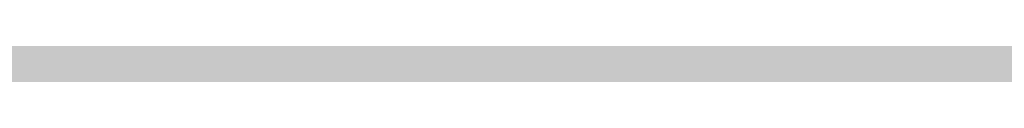
# Model space of a CAD drawing. Units: inches. Extents: x 2091 to 2899, y 967 to 2217.
# Tile 199 of 256: x 2203.18039 to 2203.25707, y 1152.24874 to 1152.25042. Entities that reach past the tile are written whole.
import ezdxf

# ---------------------------------------------------------------- set-up
doc = ezdxf.new("R2010")
doc.units = ezdxf.units.IN
doc.layers.add('A-WALL-PATT', color=141, linetype='Continuous', lineweight=13, true_color=0xadddf7)

msp = doc.modelspace()

# ---------------------------------------------------------------- hatches: boundary and pattern name
at = {"layer": 'A-WALL-PATT'}
h = msp.add_hatch(color=256, dxfattribs=at)
h.dxf.hatch_style = 1
h.paths.add_polyline_path([(2803.143603, 2050.919059), (2203.143603, 2050.919059), (2203.143603, 1090.919059), (2803.143603, 1090.919059)])
h.paths.add_polyline_path([(2635.79885, 1147.540465), (2674.524052, 1147.540465, 0.376086), (2678.529665, 1152.880202), (2678.529665, 1159.556473, 0.333335), (2674.524319, 1163.561846), (2674.524319, 1163.56185), (2674.524319, 1192.93439), (2635.805971, 1192.93439), (2597.087622, 1192.93439), (2597.087622, 1163.561846, 0.333335), (2593.082276, 1159.556473), (2593.082276, 1152.880202, 0.376086), (2597.087889, 1147.540465)], flags=0)
h.paths.add_polyline_path([(2436.010433, 1278.240778, 0.000483), (2435.952643, 1278.215027, -0.001328), (2435.935625, 1278.111693, -0.001711), (2436.11644, 1278.040758, 0.002185)], flags=0)
h.paths.add_polyline_path([(2794.143603, 1143.419059), (2794.143603, 1347.419059), (2543.370171, 1347.419059), (2543.370171, 1351.919059), (2794.143603, 1351.919059), (2794.143603, 1392.713555), (2793.947398, 1392.713555), (2793.947398, 1473.5369), (2794.143603, 1473.5369), (2794.143603, 1531.919059), (2650.143603, 1531.919059), (2650.143603, 1536.419059), (2794.143603, 1536.419059), (2794.143603, 1692.419059), (2609.375609, 1692.419059), (2609.375609, 1644.419059), (2604.875609, 1644.419059), (2604.875609, 1744.919059), (2609.375609, 1744.919059), (2609.375609, 1696.919059), (2794.143603, 1696.919059), (2794.143603, 1780.919059), (2609.643603, 1780.919059), (2493.875609, 1780.919059), (2493.875609, 1785.419059), (2609.643603, 1785.419059), (2794.143603, 1785.419059), (2794.143603, 1847.938821), (2793.951222, 1847.938821), (2793.951222, 1928.762166), (2794.143603, 1928.762166), (2794.143603, 1941.419059), (2614.143603, 1941.419059), (2614.143603, 1821.419059), (2609.643603, 1821.419059), (2609.643603, 1941.419059), (2392.143603, 1941.419059), (2392.143603, 1819.919059), (2387.643603, 1819.919059), (2387.643603, 1941.419059), (2212.143603, 1941.419059), (2212.143603, 1783.919059), (2392.143603, 1783.919059), (2392.143603, 1780.919059), (2212.143603, 1780.919059), (2212.143603, 1629.419059), (2387.643603, 1629.419059), (2387.643603, 1744.919059), (2392.143603, 1744.919059), (2392.143603, 1627.919059), (2317.143603, 1627.919059), (2317.143603, 1551.419059), (2317.143603, 1536.419059), (2459.383591, 1536.419059), (2459.383591, 1602.39648), (2463.883591, 1602.39648), (2463.883591, 1531.919059), (2456.643603, 1531.919059), (2456.643603, 1529.919059), (2452.143603, 1529.919059), (2452.143603, 1531.919059), (2312.643603, 1531.919059), (2312.643603, 1551.419059), (2306.143603, 1551.419059), (2306.143603, 1555.919059), (2308.143603, 1555.919059), (2308.143603, 1551.419059), (2312.643603, 1551.419059), (2312.643603, 1627.919059), (2212.143603, 1627.919059), (2212.143603, 1555.919059), (2270.143603, 1555.919059), (2270.143603, 1551.419059), (2212.143603, 1551.419059), (2212.143603, 1351.919059), (2272.143603, 1351.919059), (2272.143603, 1347.419059), (2212.143603, 1347.419059), (2212.143603, 1275.419059), (2308.143603, 1275.419059), (2308.143603, 1351.919059), (2452.143603, 1351.919059), (2452.143603, 1493.919059), (2456.643603, 1493.919059), (2456.643603, 1347.419059), (2312.643603, 1347.419059), (2312.643603, 1270.919059), (2212.143603, 1270.919059), (2212.143603, 1099.919059), (2281.237523, 1099.919059), (2282.871041, 1110.913803), (2282.008341, 1116.996603), (2278.557741, 1121.420403), (2268.205641, 1128.056203), (2272.087641, 1128.056203), (2273.812941, 1131.927003), (2279.420341, 1134.691903), (2285.027841, 1135.244903), (2287.615841, 1137.456803), (2288.047141, 1138.009803), (2289.341141, 1140.774703), (2291.066541, 1139.668703), (2292.360541, 1135.244903), (2295.379841, 1136.903803), (2296.242541, 1135.797903), (2297.105241, 1133.033003), (2300.124641, 1138.009803), (2303.143941, 1138.009803), (2304.437941, 1135.797903), (2303.143941, 1133.586003), (2306.594641, 1134.691903), (2307.888741, 1133.033003), (2310.908041, 1135.244903), (2313.927441, 1134.138903), (2315.62686, 1132.427102), (2308.320041, 1117.549603), (2290.203841, 1109.807903), (2288.909841, 1103.172103), (2289.272309, 1099.919059), (2434.918227, 1099.919059), (2431.593227, 1124.788059), (2429.930227, 1169.553059), (2430.927185, 1240.519694), (2435.658926, 1238.186126), (2437.135227, 1196.554059), (2438.798227, 1143.973059), (2442.678227, 1111.998059), (2446.558227, 1099.919059), (2794.143603, 1099.919059), (2794.143603, 1138.919059), (2548.032447, 1138.919059), (2548.032447, 1143.419059), (2548.032447, 1148.819059), (2546.668457, 1148.031559), (2528.685692, 1179.178622, 0.256256), (2512.032447, 1148.819059), (2512.032447, 1143.419059), (2512.032447, 1138.919059), (2507.532447, 1138.919059), (2507.532447, 1143.419059), (2507.532447, 1148.819059, 0.256256), (2490.879202, 1179.178622), (2472.896437, 1148.031559), (2471.532447, 1148.819059), (2471.532447, 1143.419059), (2467.032447, 1143.419059), (2467.032447, 1269.945786, 0.039061), (2460.909987, 1273.580059), (2467.032447, 1273.580059), (2467.032447, 1286.325364, 0.014511), (2465.216194, 1286.761905), (2467.032447, 1287.052576), (2467.032447, 1323.419059), (2471.532447, 1323.419059), (2471.532447, 1148.819059), (2489.532447, 1179.995973), (2490.896437, 1179.208473), (2490.879202, 1179.178622, -0.256256), (2507.532447, 1148.819059), (2507.532447, 1143.419059), (2512.032447, 1143.419059), (2512.032447, 1148.819059, -0.256256), (2528.685692, 1179.178622), (2528.668457, 1179.208473), (2530.032447, 1179.995973), (2548.032447, 1148.819059), (2548.032447, 1143.419059)], flags=16)
h.paths.add_polyline_path([(2607.768546, 1200.945083), (2607.768546, 1265.030625), (2597.087622, 1281.052011), (2619.784585, 1281.052011), (2627.795278, 1337.12686), (2635.79885, 1337.12686), (2643.816663, 1337.12686), (2651.827356, 1281.052011), (2674.524319, 1281.052011), (2663.843395, 1265.030625), (2663.843395, 1200.945083), (2635.805971, 1200.945083)], flags=0)
edge = h.paths.add_edge_path(flags=0)
edge.add_ellipse((13303.896215, 1272.998725), major_axis=(-10595.31304, 0.000001), ratio=0.842303870086, start_angle=0.6282372191, end_angle=0.6465540999, ccw=False)
edge.add_ellipse((2711.70045, 1156.852678), major_axis=(2.219769, 0), ratio=0.84230387, start_angle=111.535244, end_angle=180.628237, ccw=False)
edge.add_ellipse((13303.156292, 1272.998725), major_axis=(-10593.026306, 0), ratio=0.842303869544, start_angle=0.5282714718, end_angle=0.6465540971, ccw=False)
edge.add_line((2710.764596, 1175.333295), (2710.129986, 1175.333295))
edge.add_ellipse((2710.129986, 1176.579775), major_axis=(1.479846, 0), ratio=0.84230387, start_angle=180, end_angle=270, ccw=False)
edge.add_line((2708.65014, 1176.579775), (2708.65014, 1200.782914))
edge.add_ellipse((2710.129986, 1200.782914), major_axis=(1.479846, 0), ratio=0.84230387, start_angle=90, end_angle=180, ccw=False)
edge.add_line((2710.129986, 1202.029394), (2710.465075, 1202.029394))
edge.add_ellipse((13303.156292, 1272.998725), major_axis=(-10593.026306, 0), ratio=0.842303869544, start_angle=-0.0902290886, end_angle=0.3838667788, ccw=False)
edge.add_ellipse((2710.129986, 1290.927031), major_axis=(-1.479846, 0), ratio=0.84230387, start_angle=0, end_angle=90, ccw=False)
edge.add_line((2708.65014, 1290.927031), (2708.65014, 1315.13017))
edge.add_ellipse((2710.129986, 1315.13017), major_axis=(-1.479846, 0), ratio=0.84230387, start_angle=-90, end_angle=0, ccw=False)
edge.add_line((2710.129986, 1316.37665), (2710.706314, 1316.37665))
edge.add_ellipse((3238.40172, 1296.289566), major_axis=(528.234, 0), ratio=0.8423038695, start_angle=176.34957241, end_angle=177.82004969, ccw=False)
edge.add_ellipse((2775.063043, 1071.450696), major_axis=(313.307761, 0), ratio=0.8423038695, start_angle=102.12596555, end_angle=103.78052899, ccw=False)
edge.add_ellipse((2775.063043, 1078.305698), major_axis=(-305.302891, 0), ratio=0.8423038695, start_angle=-79.790461, end_angle=-77.55537271, ccw=False)
edge.add_ellipse((2695.141767, 1541.975383), major_axis=(-250.960216, 0), ratio=0.8423038695, start_angle=99.25656601, end_angle=102.55493264)
edge.add_line((2741.410326, 1334.214255), (2747.132545, 1337.378477))
edge.add_ellipse((2747.538616, 1336.857478), major_axis=(-0.739923, 0), ratio=0.8423039, start_angle=270, end_angle=307.93313, ccw=False)
edge.add_ellipse((2747.538616, 1336.857478), major_axis=(-0.739923, 0), ratio=0.8423039, start_angle=232.06687, end_angle=270, ccw=False)
edge.add_line((2747.944687, 1337.378477), (2753.666906, 1334.214255))
edge.add_ellipse((2799.935466, 1541.975383), major_axis=(250.960216, 0), ratio=0.8423038695, start_angle=257.44506736, end_angle=260.74343399)
edge.add_ellipse((2720.014189, 1078.305698), major_axis=(305.302891, 0), ratio=0.8423038695, start_angle=77.55537271, end_angle=79.790461, ccw=False)
edge.add_ellipse((2720.014189, 1071.450696), major_axis=(-313.307761, 0), ratio=0.8423038695, start_angle=256.21947101, end_angle=257.87403445, ccw=False)
edge.add_ellipse((2256.675512, 1296.289566), major_axis=(-528.234, 0), ratio=0.8423038695, start_angle=182.17995031, end_angle=183.65042759, ccw=False)
edge.add_line((2784.370918, 1316.37665), (2784.947247, 1316.37665))
edge.add_ellipse((2784.947247, 1315.13017), major_axis=(1.479846, 0), ratio=0.84230387, start_angle=0, end_angle=90, ccw=False)
edge.add_line((2786.427093, 1315.13017), (2786.427093, 1290.927031))
edge.add_ellipse((2784.947247, 1290.927031), major_axis=(1.479846, 0), ratio=0.84230387, start_angle=270, end_angle=360, ccw=False)
edge.add_ellipse((-7808.07906, 1272.998725), major_axis=(10593.026306, 0), ratio=0.842303869544, start_angle=-0.3838667788, end_angle=0.0902290886, ccw=False)
edge.add_line((2784.612157, 1202.029394), (2784.947247, 1202.029394))
edge.add_ellipse((2784.947247, 1200.782914), major_axis=(1.479846, 0), ratio=0.84230387, start_angle=0, end_angle=90, ccw=False)
edge.add_line((2786.427093, 1200.782914), (2786.427093, 1176.579775))
edge.add_ellipse((2784.947247, 1176.579775), major_axis=(-1.479846, 0), ratio=0.84230387, start_angle=90, end_angle=180, ccw=False)
edge.add_line((2784.947247, 1175.333295), (2784.312636, 1175.333295))
edge.add_ellipse((-7808.07906, 1272.998725), major_axis=(10593.026306, 0), ratio=0.842303869544, start_angle=-0.6186431963, end_angle=-0.5282714718, ccw=False)
edge.add_ellipse((2783.376783, 1156.852678), major_axis=(-2.219769, 0), ratio=0.84230387, start_angle=179.371763, end_angle=248.464757, ccw=False)
edge.add_ellipse((-7808.818983, 1272.998725), major_axis=(-10595.31304, 0.000004), ratio=0.842303865762, start_angle=179.3534459226, end_angle=179.3717628034, ccw=False)
edge.add_ellipse((2780.297303, 1153.500793), major_axis=(-5.246426, 0), ratio=0.84230387, start_angle=90, end_angle=179.353446, ccw=False)
edge.add_line((2780.297303, 1149.081708), (2714.77993, 1149.081708))
edge.add_ellipse((2714.77993, 1153.500793), major_axis=(5.246426, 0), ratio=0.84230387, start_angle=180.646554, end_angle=270, ccw=False)
edge = h.paths.add_edge_path(flags=0)
edge.add_line((2718.187367, 1151.007833), (2718.187367, 1170.472364))
edge.add_ellipse((2721.14706, 1170.472364), major_axis=(-2.959692, 0), ratio=0.84230387, start_angle=-90, end_angle=0, ccw=False)
edge.add_line((2721.14706, 1172.965324), (2773.930173, 1172.965324))
edge.add_ellipse((2773.930173, 1170.472364), major_axis=(-2.959692, 0), ratio=0.84230387, start_angle=180, end_angle=270, ccw=False)
edge.add_line((2776.889865, 1170.472364), (2776.889865, 1151.007833))
edge.add_line((2776.889865, 1151.007833), (2718.187367, 1151.007833))
edge = h.paths.add_edge_path(flags=0)
edge.add_line((2718.187367, 1180.23415), (2718.187367, 1199.057834))
edge.add_ellipse((2747.538616, 1320.39864), major_axis=(147.017924, 0), ratio=0.8423038695, start_angle=256.40186531, end_angle=283.59813469)
edge.add_line((2776.889865, 1199.057834), (2776.889865, 1180.23415))
edge.add_ellipse((2747.538616, 1301.574956), major_axis=(147.017924, 0), ratio=0.8423038695, start_angle=256.40186531, end_angle=283.59813469, ccw=False)
edge = h.paths.add_edge_path(flags=0)
edge.add_ellipse((13303.156292, 1272.998725), major_axis=(-10591.54646, 0), ratio=0.842303869555, start_angle=0.0555943135, end_angle=0.3777641939, ccw=False)
edge.add_line((2711.616859, 1262.72171), (2715.667408, 1249.495396))
edge.add_ellipse((6413.891963, 1241.691919), major_axis=(-3698.236159, 0), ratio=0.84230386955, start_angle=-0.120897369, end_angle=0.364076349)
edge.add_line((2715.761038, 1218.192455), (2711.934307, 1203.167361))
edge = h.paths.add_edge_path(flags=0)
edge.add_line((2718.187367, 1251.074566), (2716.002485, 1267.450435))
edge.add_ellipse((2742.151175, 1202.18954), major_axis=(81.772585, 0), ratio=0.84230387, start_angle=94.27742096, end_angle=111.8349538, ccw=False)
edge.add_line((2737.009748, 1270.930626), (2758.067484, 1270.930626))
edge.add_ellipse((2752.926058, 1202.18954), major_axis=(81.772585, 0), ratio=0.84230387, start_angle=68.1650462, end_angle=85.72257904, ccw=False)
edge.add_line((2779.074747, 1267.450435), (2776.889865, 1251.074566))
edge.add_ellipse((2750.338059, 1187.885356), major_axis=(79.579664, 0), ratio=0.84230387, start_angle=67.20808512, end_angle=85.1299304)
edge.add_line((2756.034656, 1254.743656), (2739.042576, 1254.743656))
edge.add_ellipse((2744.739174, 1187.885356), major_axis=(79.579664, 0), ratio=0.84230387, start_angle=94.8700696, end_angle=112.79191488)
edge = h.paths.add_edge_path(flags=0)
edge.add_line((2783.142926, 1203.167361), (2779.316194, 1218.192455))
edge.add_ellipse((-918.81473, 1241.691919), major_axis=(3698.236159, 0), ratio=0.84230386955, start_angle=-0.364076349, end_angle=0.120897369)
edge.add_line((2779.409825, 1249.495396), (2783.460373, 1262.72171))
edge.add_ellipse((-7808.07906, 1272.998725), major_axis=(-10591.54646, 0), ratio=0.84230386954, start_angle=179.6222358061, end_angle=179.9444056865, ccw=False)
edge = h.paths.add_edge_path(flags=0)
edge.add_ellipse((2734.200892, 1286.69044), major_axis=(-0.356609, 6.340078), ratio=0.60383358, start_angle=89.0020143, end_angle=253.657408, ccw=False)
edge.add_line((2730.369001, 1286.541806), (2730.369001, 1301.35198))
edge.add_line((2730.369001, 1301.35198), (2735.913311, 1305.214803))
edge.add_ellipse((2736.384917, 1304.734561), major_axis=(0.739923, 0), ratio=0.8423039, start_angle=90, end_angle=134.480211, ccw=False)
edge.add_line((2736.384917, 1305.357801), (2738.032783, 1305.357801))
edge.add_line((2738.032783, 1305.357801), (2738.032783, 1307.707927))
edge.add_ellipse((2794.201642, 1307.707927), major_axis=(56.168859, 0), ratio=0.84230387, start_angle=150.5614304, end_angle=180, ccw=False)
edge.add_ellipse((2700.875591, 1307.707927), major_axis=(-56.168859, 0), ratio=0.84230387, start_angle=180, end_angle=209.4385696, ccw=False)
edge.add_line((2757.04445, 1307.707927), (2757.04445, 1305.357801))
edge.add_line((2757.04445, 1305.357801), (2758.692316, 1305.357801))
edge.add_ellipse((2758.692316, 1304.734561), major_axis=(-0.739923, 0), ratio=0.8423039, start_angle=225.519789, end_angle=270, ccw=False)
edge.add_line((2759.163922, 1305.214803), (2764.708231, 1301.35198))
edge.add_line((2764.708231, 1301.35198), (2764.708231, 1286.541806))
edge.add_ellipse((2760.87634, 1286.69044), major_axis=(0.356609, 6.340078), ratio=0.60383358, start_angle=106.342592, end_angle=270.9979857, ccw=False)
edge.add_line((2757.04445, 1285.79709), (2757.04445, 1307.707927))
edge.add_ellipse((2700.875591, 1307.707927), major_axis=(-56.168859, 0), ratio=0.84230387, start_angle=180, end_angle=209.4385696)
edge.add_ellipse((2794.201642, 1307.707927), major_axis=(56.168859, 0), ratio=0.84230387, start_angle=150.5614304, end_angle=180)
edge.add_line((2738.032783, 1307.707927), (2738.032783, 1285.79709))
h.paths.add_polyline_path([(2417.812273, 1104.449704), (2413.492273, 1102.529704), (2410.612273, 1103.969704), (2409.172273, 1106.369704), (2407.252273, 1107.329704), (2406.292273, 1109.729704), (2405.332273, 1114.049704), (2405.332273, 1117.889704), (2406.292273, 1120.129704), (2407.252273, 1119.809704), (2408.848322, 1118.327658), (2410.173945, 1119.42417), (2410.211273, 1120.405704), (2411.040731, 1121.419054), (2410.699273, 1119.858704), (2410.173945, 1119.42417), (2410.088452, 1117.176109), (2411.132836, 1116.206324), (2413.972273, 1119.329704), (2416.852273, 1120.769704), (2416.869721, 1120.798784), (2417.035071, 1119.405116), (2417.896213, 1118.143384), (2418.292273, 1118.369704), (2419.544447, 1120.039269), (2419.360915, 1118.387487), (2419.032108, 1119.356151), (2418.398939, 1118.511926), (2419.252273, 1114.529704), (2418.794091, 1107.198795)], flags=0)
h.paths.add_polyline_path([(2508.870171, 1347.419059), (2508.370171, 1347.419059), (2508.370171, 1351.919059), (2508.870171, 1351.919059)], flags=0)
h.paths.add_polyline_path([(2473.370171, 1347.419059), (2472.370171, 1347.419059), (2467.870171, 1347.419059), (2467.870171, 1455.419059), (2472.370171, 1455.419059), (2472.370171, 1352.419059), (2473.370171, 1352.419059)], flags=0)
h.paths.add_polyline_path([(2352.106244, 1217.446197), (2349.226244, 1218.886197), (2347.786244, 1221.286197), (2345.866244, 1222.246197), (2344.906244, 1224.646197), (2343.946244, 1228.966197), (2343.946244, 1232.806197), (2344.906244, 1235.046197), (2345.866244, 1234.726197), (2347.462293, 1233.244152), (2348.787916, 1234.340663), (2348.825244, 1235.322197), (2349.654702, 1236.335547), (2349.313244, 1234.775197), (2348.787916, 1234.340663), (2348.702423, 1232.092603), (2349.746807, 1231.122817), (2352.586244, 1234.246197), (2355.466244, 1235.686197), (2355.483692, 1235.715277), (2355.649043, 1234.321609), (2356.510185, 1233.059877), (2356.906244, 1233.286197), (2358.158418, 1234.955762), (2357.974887, 1233.30398), (2357.646079, 1234.272644), (2357.012911, 1233.428419), (2357.866244, 1229.446197), (2357.408062, 1222.115288), (2356.426244, 1219.366197)], flags=0)
h.paths.add_polyline_path([(2348.2968, 1112.22442), (2347.0138, 1112.31042), (2345.5298, 1114.12742), (2345.7318, 1115.85842), (2346.8118, 1116.98242), (2346.8118, 1114.64642), (2345.8668, 1114.21442), (2346.8798, 1114.30042)], flags=0)
h.paths.add_polyline_path([(2347.0138, 1110.92642), (2346.2718, 1110.49342), (2346.6098, 1111.18642)], flags=0)
h.paths.add_polyline_path([(2345.8668, 1118.19442), (2345.5298, 1117.32942), (2343.7078, 1118.02142), (2344.3828, 1118.62642)], flags=0)
h.paths.add_polyline_path([(2346.6768, 1109.28242), (2346.0698, 1108.07142), (2345.8668, 1110.06142)], flags=0)
h.paths.add_polyline_path([(2345.0568, 1119.75142), (2343.6398, 1119.75142), (2343.9778, 1121.13542)], flags=0)
h.paths.add_polyline_path([(2345.2598, 1116.55042), (2345.1248, 1115.85842), (2344.9218, 1115.68542), (2344.7198, 1116.37742)], flags=0)
h.paths.add_polyline_path([(2345.6648, 1112.31042), (2345.4618, 1111.53242), (2344.0448, 1111.96442), (2344.6518, 1112.57042)], flags=0)
h.paths.add_polyline_path([(2345.1918, 1113.34942), (2344.4498, 1113.86842), (2344.7198, 1114.38742)], flags=0)
h.paths.add_polyline_path([(2344.6518, 1116.80942), (2344.1798, 1115.68542), (2344.6518, 1115.33942), (2343.9098, 1114.90642), (2343.0328, 1115.94442), (2343.6398, 1116.46342)], flags=0)
h.paths.add_polyline_path([(2345.8668, 1106.68642), (2344.9898, 1105.56242), (2344.5168, 1106.60042)], flags=0)
h.paths.add_polyline_path([(2344.8548, 1110.06142), (2344.5168, 1109.28242), (2344.1128, 1109.71542)], flags=0)
h.paths.add_polyline_path([(2344.0448, 1113.52242), (2343.4378, 1113.08942), (2342.7628, 1113.95442)], flags=0)
h.paths.add_polyline_path([(2344.3148, 1111.01242), (2342.9648, 1110.32042), (2342.9648, 1111.09942)], flags=0)
h.paths.add_polyline_path([(2345.1248, 1104.69742), (2344.5848, 1103.74542), (2344.4498, 1104.26442)], flags=0)
h.paths.add_polyline_path([(2342.8298, 1121.22242), (2341.7498, 1120.53042), (2340.5358, 1121.04942), (2340.1308, 1121.82842), (2340.6708, 1122.95242), (2341.1428, 1121.82842), (2341.6148, 1122.00142)], flags=0)
h.paths.add_polyline_path([(2342.9648, 1119.75142), (2343.0328, 1118.45342), (2342.0878, 1118.02142), (2342.0198, 1119.49142)], flags=0)
h.paths.add_polyline_path([(2342.6948, 1116.89642), (2341.9528, 1116.63642), (2342.0198, 1117.32942)], flags=0)
h.paths.add_polyline_path([(2343.0328, 1112.22442), (2342.0198, 1111.79142), (2341.5478, 1112.22442), (2342.3578, 1113.34942)], flags=0)
h.paths.add_polyline_path([(2343.7748, 1104.43742), (2342.6278, 1102.88042), (2342.6948, 1104.61042), (2343.4378, 1105.12942)], flags=0)
h.paths.add_polyline_path([(2342.0198, 1115.07942), (2340.8058, 1115.51242), (2340.9408, 1116.37742)], flags=0)
h.paths.add_polyline_path([(2341.4808, 1120.09742), (2341.4808, 1119.40542), (2341.0758, 1119.57842), (2341.1428, 1120.09742)], flags=0)
h.paths.add_polyline_path([(2341.8178, 1114.47342), (2340.9408, 1113.08942), (2340.8058, 1114.56042)], flags=0)
h.paths.add_polyline_path([(2341.1428, 1118.54042), (2340.9408, 1116.98242), (2339.0508, 1117.67542), (2339.0508, 1118.62642)], flags=0)
h.paths.add_polyline_path([(2342.6948, 1101.66842), (2341.9528, 1101.84142), (2342.5598, 1102.36142)], flags=0)
h.paths.add_polyline_path([(2340.3328, 1119.66542), (2338.4438, 1119.57842), (2337.9038, 1120.35742), (2339.6578, 1120.61642)], flags=0)
h.paths.add_polyline_path([(2340.3328, 1115.33942), (2340.0628, 1113.69542), (2339.3878, 1115.33942)], flags=0)
h.paths.add_polyline_path([(2341.8178, 1103.83142), (2341.5478, 1102.88042), (2341.1428, 1103.65842)], flags=0)
h.paths.add_polyline_path([(2339.0508, 1122.86642), (2337.2958, 1121.82842), (2337.0938, 1123.12542), (2337.7688, 1123.81842)], flags=0)
h.paths.add_polyline_path([(2339.1178, 1121.74142), (2338.8478, 1121.22242), (2338.1738, 1121.04942), (2338.3758, 1121.56842)], flags=0)
h.paths.add_polyline_path([(2339.1858, 1119.31942), (2338.6458, 1118.71342), (2338.2408, 1118.10742), (2338.2408, 1118.88642)], flags=0)
h.paths.add_polyline_path([(2341.1428, 1101.92842), (2340.6028, 1101.23642), (2340.0628, 1101.84142), (2340.6028, 1102.36142)], flags=0)
h.paths.add_polyline_path([(2337.6338, 1117.76142), (2336.6208, 1118.28042), (2337.2958, 1118.97242)], flags=0)
h.paths.add_polyline_path([(2336.8238, 1119.57842), (2334.7988, 1118.97242), (2335.2038, 1120.35742), (2336.5538, 1120.87642)], flags=0)
h.paths.add_polyline_path([(2339.1178, 1100.45742), (2337.3638, 1100.54342), (2336.7558, 1101.23642)], flags=0)
h.paths.add_polyline_path([(2336.3508, 1122.43342), (2336.0138, 1121.91442), (2334.9338, 1122.43342), (2334.5288, 1123.47142), (2335.7438, 1122.77942)], flags=0)
h.paths.add_polyline_path([(2334.7318, 1120.87642), (2334.2588, 1120.35742), (2334.0568, 1120.78942), (2334.5968, 1121.30842)], flags=0)
h.paths.add_polyline_path([(2334.4618, 1122.17442), (2332.5718, 1121.30842), (2331.3568, 1122.17442), (2332.0998, 1122.86642)], flags=0)
h.paths.add_polyline_path([(2334.2588, 1118.54042), (2333.3818, 1118.45342), (2333.6518, 1119.31942)], flags=0)
h.paths.add_polyline_path([(2335.5418, 1102.27442), (2334.1918, 1102.62042), (2335.2718, 1103.31242)], flags=0)
h.paths.add_polyline_path([(2332.7068, 1119.66542), (2331.6948, 1120.44342), (2332.5048, 1120.78942)], flags=0)
h.paths.add_polyline_path([(2334.7318, 1101.14942), (2333.5168, 1101.58242), (2333.9888, 1101.75542)], flags=0)
h.paths.add_polyline_path([(2332.6398, 1116.63642), (2331.0868, 1116.29042), (2331.9648, 1118.19442)], flags=0)
h.paths.add_polyline_path([(2330.7498, 1121.56842), (2330.2768, 1120.27042), (2328.5228, 1119.31942), (2328.9948, 1121.04942)], flags=0)
h.paths.add_polyline_path([(2330.7498, 1118.62642), (2330.0078, 1117.50242), (2329.8728, 1118.02142)], flags=0)
h.paths.add_polyline_path([(2332.0998, 1102.36142), (2330.5468, 1102.01442), (2331.6948, 1102.96642)], flags=0)
h.paths.add_polyline_path([(2329.5348, 1113.60842), (2329.0628, 1112.31042), (2328.5898, 1113.34942)], flags=0)
h.paths.add_polyline_path([(2328.3878, 1117.84842), (2327.5098, 1116.55042), (2327.1728, 1117.76142)], flags=0)
h.paths.add_polyline_path([(2329.7378, 1106.51342), (2329.5348, 1105.30242), (2328.2528, 1106.08142)], flags=0)
h.paths.add_polyline_path([(2328.6578, 1114.38742), (2328.0498, 1114.12742), (2328.3198, 1114.90642)], flags=0)
h.paths.add_polyline_path([(2328.3198, 1112.22442), (2327.1058, 1112.13742), (2326.7008, 1112.65642)], flags=0)
h.paths.add_polyline_path([(2326.9028, 1115.25242), (2326.7008, 1114.12742), (2325.2158, 1113.60842), (2326.0928, 1115.33942)], flags=0)
h.paths.add_polyline_path([(2326.6328, 1108.33042), (2326.0928, 1107.37942), (2325.8908, 1108.50342), (2326.4978, 1109.10942)], flags=0)
h.paths.add_polyline_path([(2615.143603, 1531.919059), (2609.643603, 1531.919059), (2609.643603, 1620.419059), (2614.143603, 1620.419059), (2614.143603, 1536.419059), (2615.143603, 1536.419059)], flags=0)
h.paths.add_polyline_path([(2545.143603, 1563.419059), (2464.143603, 1563.419059), (2464.143603, 1632.419059), (2509.143603, 1632.419059), (2509.143603, 1627.919059), (2509.143603, 1603.919059), (2468.643603, 1603.919059), (2468.643603, 1567.919059), (2540.643603, 1567.919059), (2540.643603, 1591.919059), (2545.143603, 1591.919059)], flags=0)
h.paths.add_polyline_path([(2388.969048, 1549.985735), (2357.434181, 1549.985735), (2357.434181, 1623.360778), (2399.362777, 1623.360778), (2435.689465, 1623.360778), (2435.592547, 1602.559273), (2435.592547, 1602.39648), (2388.969048, 1602.39648)], flags=0)
h.paths.add_polyline_path([(2388.880628, 1555.809151), (2374.904429, 1555.809151), (2374.904429, 1600.571564), (2374.904429, 1615.457645), (2406.350877, 1615.457645), (2406.350877, 1618.939431), (2412.174293, 1615.457645), (2406.350877, 1611.97586), (2406.350877, 1615.457645), (2388.880628, 1615.457645)], flags=0)
h.paths.add_polyline_path([(2568.875609, 1644.419059), (2453.375609, 1644.419059), (2453.375609, 1785.419059), (2457.875609, 1785.419059), (2457.875609, 1648.919059), (2568.875609, 1648.919059)], flags=0)
h.paths.add_polyline_path([(2212.143603, 1945.919059), (2212.143603, 2041.919059), (2794.143603, 2041.919059), (2794.143603, 1945.919059)], flags=16)
h.paths.add_polyline_path([(2271.082728, 1964.317238), (2776.852968, 1964.317238), (2776.852968, 2037.169623), (2271.082728, 2037.169623)], flags=8)
h.paths.add_polyline_path([(2380.649285, 1536.824144), (2461.040809, 1536.824144), (2461.040809, 1554.652587), (2380.649285, 1554.652587)], flags=8)
h.paths.add_polyline_path([(2240.755709, 1609.725451), (2309.185829, 1609.725451), (2309.185829, 1617.698204), (2240.755709, 1617.698204)], flags=8)
h.paths.add_polyline_path([(2212.677255, 1313.504102), (2282.59152, 1313.504102), (2282.59152, 1322.745239), (2212.677255, 1322.745239)], flags=8)
h.paths.add_polyline_path([(2457.111976, 1114.778574), (2558.481581, 1114.778574), (2558.481581, 1142.219682), (2457.111976, 1142.219682)], flags=8)
h.paths.add_polyline_path([(2473.442337, 1273.010067), (2604.641226, 1273.010067), (2604.641226, 1318.346935), (2473.442337, 1318.346935)], flags=8)
h.paths.add_polyline_path([(2638.876302, 1626.977432), (2684.250367, 1627.976738), (2684.038483, 1637.597494), (2638.664417, 1636.598188)], flags=8)
h.paths.add_polyline_path([(2537.590554, 1453.793447), (2628.389547, 1453.793447), (2628.389547, 1475.344811), (2537.590554, 1475.344811)], flags=8)
h.paths.add_polyline_path([(2504.137638, 1714.632397), (2554.647187, 1714.632397), (2554.647187, 1730.237712), (2504.137638, 1730.237712)], flags=8)
h.paths.add_polyline_path([(2487.501181, 1575.651872), (2535.097121, 1575.651872), (2535.097121, 1598.377646), (2487.501181, 1598.377646)], flags=8)
h.paths.add_polyline_path([(2709.0994, 1735.710278), (2740.016601, 1735.710278), (2740.016601, 1749.937641), (2709.0994, 1749.937641)], flags=8)
h.paths.add_polyline_path([(2442.438424, 1792.171657), (2564.728835, 1792.171657), (2564.728835, 1842.000163), (2442.438424, 1842.000163)], flags=8)
h.paths.add_polyline_path([(2655.815801, 1809.644076), (2789.520142, 1806.693796), (2790.084977, 1832.291638), (2656.380635, 1835.241918)], flags=8)
h.paths.add_polyline_path([(2234.842697, 1797.720143), (2368.592851, 1794.768852), (2369.160718, 1820.504132), (2235.410564, 1823.455423)], flags=8)
h.paths.add_polyline_path([(2245.138466, 1644.006335), (2398.427733, 1640.6239), (2398.994842, 1666.32482), (2245.705575, 1669.707255)], flags=8)
h.paths.add_polyline_path([(2306.142847, 1431.168519), (2413.768314, 1428.793687), (2414.333148, 1454.391529), (2306.707682, 1456.76636)], flags=8)
h.paths.add_polyline_path([(2306.834582, 1458.233145), (2393.380484, 1456.323449), (2393.932808, 1481.354358), (2307.386907, 1483.264054)], flags=8)

doc.saveas('drawing.dxf')
